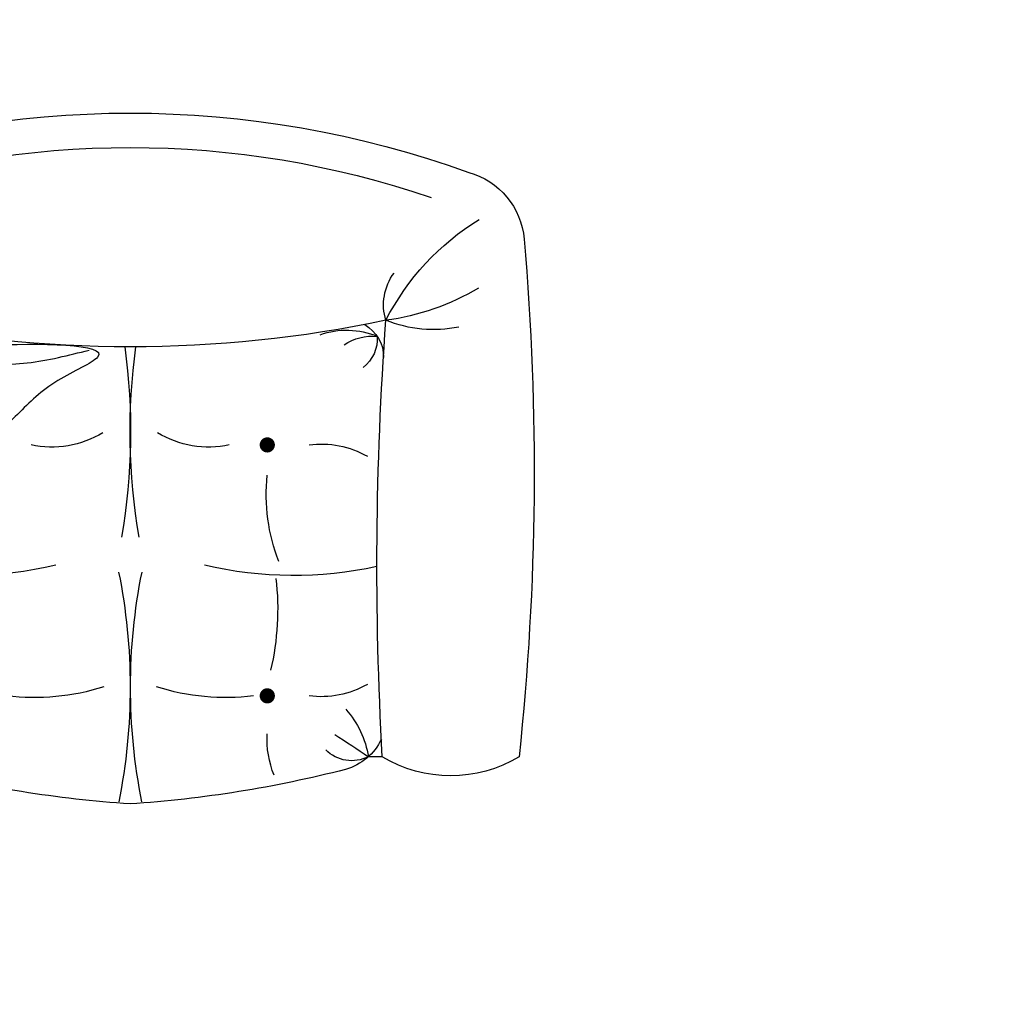
# Model space of a CAD drawing. Units: inches. Extents: x 844 to 2234, y 346 to 1084.
# Tile 23 of 93: x 1116 to 1136, y 710 to 731. Entities that reach past the tile are written whole.
import ezdxf

# ---------------------------------------------------------------- set-up
doc = ezdxf.new("R2010")
doc.units = ezdxf.units.IN
doc.header["$MEASUREMENT"] = 0
doc.layers.add('A-ANNO-DIMS', color=2, linetype='Continuous', lineweight=18)
doc.layers.add('furniture', color=8, linetype='Continuous', lineweight=18)
doc.layers.add('RA-AP-01$0$FURN', color=3, linetype='Continuous')
doc.layers.add('RA-AP-01$0$WOOD', color=64, linetype='Continuous')
doc.styles.get("Standard").update_dxf_attribs({"font": 'arial.ttf'})
doc.dimstyles.get("Standard").update_dxf_attribs({"dimtxt": 6, "dimasz": 3, "dimexe": 0.18, "dimexo": 0.0625, "dimgap": 0.09, "dimtad": 0, "dimtih": 1, "dimtoh": 1, "dimdec": 1, "dimzin": 0, "dimdsep": 46, "dimlunit": 3, "dimtxsty": 'Standard', "dimblk": 'ARCHTICK', "dimcen": 0.09, "dimadec": 0, "dimazin": 0, "dimtfac": 1, "dimtdec": 1, "dimtofl": 0, "dimtmove": 0, "dimatfit": 3, "dimfxl": 1, "dimtolj": 1, "dimtzin": 0, "dimarcsym": 0})

# ---------------------------------------------------------------- blocks, each defined once
blk = doc.blocks.new('A$C7F4351E2')
at = {"layer": 'RA-AP-01$0$FURN'}
for p, q in [((8.352559572600457, -8.263941955512525), (8.35255957259913, -8.282283310927069)), ((8.352559572600457, -8.927748273106442), (8.35255957259913, -8.909406917691898))]:
    blk.add_line(p, q, dxfattribs=at)
at = {"layer": 'RA-AP-01$0$FURN', "const_width": 0.01}
for points in [[(8.437812509519787, -8.415359762755768, 1), (8.427812509519786, -8.415359762755742, 1)], [(8.758197489244363, -8.415359762756214, -1), (8.768197489244365, -8.415359762756214, -1)], [(8.437812509519787, -8.776330465863198, -1), (8.427812509519786, -8.776330465863225, -1)], [(8.758197489244363, -8.776330465862753, 1), (8.768197489244365, -8.776330465862753, 1)]]:
    blk.add_lwpolyline(points, format="xyb", close=True, dxfattribs=at)
at = {"layer": 'RA-AP-01$0$FURN'}
for centre, radius, start, end in [((8.727559572604601, -11.61690445537682), 3.552808610866049, 85.0473312316413, 96.05887237565803), ((8.50205957259015, -8.17394195551301), 0.1744999999876311, 148.9517780040467, 211.048221995953), ((9.025650106946005, -8.176987401637472), 0.1, 15.499494600857, 85.04733123164159), ((8.77247054904813, -7.958543863781743), 0.3382138395168437, 297.2303327094027, 328.2563708342649), ((9.2484631175852, -8.302692737637487), 0.3241573581843151, 149.2985674842688, 172.3026350986055), ((7.88981694267423, -8.595845114309485), 1.310286319972027, 340.1192502251003, 19.8807497748998), ((9.084915705374858, -8.196040134964925), 0.1698955038956699, 168.877843135945, 201.8512383801196), ((7.929864357850293, -8.595845114309483), 1.224941341589781, 341.1257460634955, 18.87425393650447), ((8.947672844970796, -8.191835192646359), 0.0704710051510922, 253.1338634205325, 306.4126496157095), ((8.408522229993444, -8.33300072568355), 0.0753785023123622, 115.8745619060558, 163.9833547230034), ((8.603635103111959, -3.79706073025477), 4.473931917517753, 266.7828902523826, 274.1477233631118), ((8.878389979098333, -8.312202545234353), 0.05, 30.14777190425723, 89.99999999905349), ((10.52713941284929, -8.595845114309466), 1.634931324962266, 168.1200364254424, 191.8799635745573), ((9.101231010340802, -8.38034106221356), 0.5100538472773755, 167.6182489359307, 193.3122231353938), ((8.903279781571525, -8.31837865610295), 0.0478550828899777, 86.575295631534, 142.6833829238214), ((8.838100984994732, -8.276822957859652), 0.0683206773889159, 326.6729861493449, 5.218395042636973), ((8.810121490949696, -8.31110757721543), 0.1042084262671507, 340.4828318717155, 22.86929393278168), ((8.395364730619693, -8.304213854581548), 0.0479292786975047, 152.8070868543555, 225.4025460716553), ((8.333592787569726, -8.402663469525104), 0.1218651776285568, 48.0375529564433, 81.04623209541253), ((7.439612310514541, -8.913795367824825), 1.11020813118073, 31.93286085977143, 34.66647731879807), ((8.553131949433, -8.344109762755968), 0.1214118203512435, 150.1419074485596, 187.691663289156), ((8.642878049331348, -8.344109762756093), 0.1214118203512435, 352.3083367106845, 29.85809255128089), ((9.82633505008426, -8.696671375220811), 1.539060359583382, 165.5338783218257, 176.2437734318419), ((8.374918524725835, -8.294321202996931), 0.1212957045587361, 247.3375839744822, 273.7314750942433), ((8.546954810732721, -8.753394424755975), 0.3517162425384579, 83.41248966761125, 103.1674570565571), ((8.697701155637269, -8.172468128267624), 0.2442261434243043, 248.9017070735605, 275.9923925191661), ((8.73287643248165, -8.469775898206471), 0.3023568492824586, 173.0944825511667, 197.588060785551), ((8.889871101981017, -8.492307869305423), 0.1295083186917369, 167.9901339202812, 211.3796151021958), ((8.444145567704187, -7.829943385268752), 0.765467899454341, 258.6273206109321, 281.4174148186357), ((8.781211457338294, -7.772561243483908), 0.8232838708255751, 260.2449188973366, 277.7495311655964), ((9.82633505008426, -8.495018853398156), 1.539060359583382, 183.7562265681581, 194.4661216781742), ((8.444145567704187, -9.361312955433425), 0.765467899454341, 78.58258518136427, 101.3726793890678), ((8.781211457338294, -9.418695097218269), 0.8232838708255751, 82.25060502413102, 99.75508110266344), ((8.73287643248165, -8.721914330412496), 0.3023568492824586, 162.411939214449, 186.9055174488332), ((8.889871101981017, -8.699382359313544), 0.1295083186917369, 148.6203848978042, 192.0098660797188), ((9.101231010340802, -8.811349166405407), 0.5100538472773755, 166.6877768646062, 192.3817510640693), ((8.799643412436344, -8.749969313933361), 0.0689028341546707, 265.5384273543114, 353.5804828909086), ((8.374918524725835, -8.897369025622035), 0.1212957045587361, 86.26852490575668, 112.6624160255178), ((8.546954810732721, -8.438295803862992), 0.3517162425384579, 256.8325429434429, 276.5875103323888), ((8.697701155637269, -9.019222100351342), 0.2442261434243043, 84.00760748083387, 111.0982929264395), ((8.553131949433, -8.847580465862999), 0.1214118203512435, 172.308336710844, 209.8580925514404), ((8.785133372574222, -8.874256642962408), 0.0310151388417235, 42.62105484496073, 114.2239681486109), ((8.810121490949696, -8.880582651403534), 0.1042084262671507, 337.1307060672183, 19.51716812828453), ((8.395364730619693, -8.88747637403742), 0.0479292786975047, 134.5974539283447, 207.1929131456445), ((7.439612310514541, -8.277894860794142), 1.11020813118073, 325.333522681202, 328.0671391402286), ((8.838100984994732, -8.914867270759315), 0.0683206773889159, 354.781604957363, 33.32701385065517), ((8.408522229993444, -8.858689502935416), 0.0753785023123622, 196.0166452769965, 244.1254380939442), ((8.333592787569726, -8.789026759093863), 0.1218651776285568, 278.9537679045875, 311.9624470435567), ((8.642878049331348, -8.847580465862874), 0.1214118203512435, 330.1419074487191, 340.3913536181062), ((8.903279781571525, -8.873311572516016), 0.0478550828899777, 217.3166170761785, 273.424704368466), ((8.878389979098333, -8.879487683384612), 0.05, 270.0000000009465, 337.4173275753961), ((8.50205957259015, -9.017748273105955), 0.1744999999876311, 148.9517780040469, 211.0482219959533), ((8.603635103111959, -13.39462949836419), 4.473931917517753, 85.85227663688822, 93.21710974761734), ((8.947672844970796, -8.999855035972608), 0.0704710051510922, 53.58735038429053, 106.8661365794674), ((9.084915705374858, -8.995650093654042), 0.1698955038956699, 158.1487616198804, 191.122156864055), ((8.77247054904813, -9.233146364837223), 0.3382138395168437, 31.74362916573515, 62.76966729059727), ((9.2484631175852, -8.88899749098148), 0.3241573581843151, 187.6973649013944, 210.7014325157311), ((9.025650106946005, -9.014702826981493), 0.1, 274.9526687683584, 344.500505399143), ((8.727559572604601, -5.574785773242145), 3.552808610866049, 263.941127624342, 274.9526687683587)]:
    blk.add_arc(centre, radius, start, end, dxfattribs=at)
for points, knots in [([(8.764421239581775, -8.929562504990262), (8.755250524728652, -8.881106864374377), (8.74196437992213, -8.810906376383404), (8.80604948961138, -8.740469753734786), (8.847474678848357, -8.701097198289744), (8.897142214037096, -8.58322730303861), (8.897091569728207, -8.784804210134517), (8.88612504526093, -8.897825917224484), (8.806539053396843, -8.9185794820093), (8.764421239581775, -8.92956250499026)], [0, 0, 0, 0, 0.1367586589314792, 0.1981301758052368, 0.2677729570689282, 0.3281194902553322, 0.4737578340741565, 0.5765194025309516, 0.6920332287422236, 0.6920332287422236, 0.6920332287422236, 0.6920332287422236]), ([(8.764421239581775, -8.92956250499026), (8.782204778269502, -8.914603263160053), (8.821592007255505, -8.881471326160916), (8.86917941606436, -8.814322636989944), (8.867818990542759, -8.729338202119969), (8.881231406199264, -8.676770566934765), (8.888101821971249, -8.649843164808122)], [0, 0, 0, 0, 0.070018540671015, 0.1550780383534498, 0.2344491945777043, 0.3178048737568289, 0.3178048737568289, 0.3178048737568289, 0.3178048737568289])]:
    blk.add_open_spline(points, degree=3, knots=knots, dxfattribs=at)
blk = doc.blocks.new('A$C5D2F253E')
at = {"layer": 'RA-AP-01$0$WOOD', "xscale": -1, "rotation": 180}
blk.add_blockref('A$C7F4351E2', (-7.164808785335935, -7.45332973198748), dxfattribs=at)
blk = doc.blocks.new('_ArchTick')
at = {"color": 0, "linetype": 'ByBlock', "const_width": 0.15}
blk.add_lwpolyline([(-0.5, -0.5), (0.5, 0.5)], dxfattribs=at)
blk = doc.blocks.new('*D144')
at = {"layer": 'A-ANNO-DIMS', "color": 0, "lineweight": -2, "transparency": 16777216}
for p, q in [((1096.615948, 439.3732739999999), (1096.615948, 1074.743301)), ((1143.115948, 492.373274), (1143.115948, 1074.743301)), ((1096.615948, 1074.563301), (1102.481950728513, 1074.563301)), ((1143.115948, 1074.563301), (1137.249945271487, 1074.563301))]:
    blk.add_line(p, q, dxfattribs=at)
at = {"layer": 'Defpoints', "color": 0, "transparency": 16777216}
for p in [(1143.115948, 1074.563301), (1143.115948, 492.3107739999999), (1096.615948, 439.3107739999999)]:
    blk.add_point(p, dxfattribs=at)
at = {"layer": 'A-ANNO-DIMS', "color": 0, "lineweight": -2, "transparency": 16777216, "xscale": 3, "yscale": 3, "zscale": 3, "rotation": 180}
blk.add_blockref('_ArchTick', (1096.615948, 1074.563301), dxfattribs=at)
at = {"layer": 'A-ANNO-DIMS', "color": 0, "lineweight": -2, "transparency": 16777216, "xscale": 3, "yscale": 3, "zscale": 3}
blk.add_blockref('_ArchTick', (1143.115948, 1074.563301), dxfattribs=at)
at = {"layer": 'A-ANNO-DIMS', "color": 0, "transparency": 16777216, "insert": (1119.865948, 1074.563301), "char_height": 6, "attachment_point": 5}
blk.add_mtext('\\A1;3\'-10 1/2"', dxfattribs=at)

msp = doc.modelspace()

# ---------------------------------------------------------------- block references
at = {"layer": 'furniture', "xscale": 15.94108302203742, "yscale": 15.94108302203742, "zscale": 15.94108302203742, "rotation": 90}
msp.add_blockref('A$C5D2F253E', (1136.147844094663, 696.2584716700112), dxfattribs=at)

# ---------------------------------------------------------------- dimensions: what is measured, and where the dimension line sits
at = {"layer": 'A-ANNO-DIMS'}
dim = msp.add_linear_dim(base=(1143.115948, 1074.563301), p1=(1096.615948, 439.3107739999999), p2=(1143.115948, 492.3107739999999), dimstyle='Standard', override={"dimdec": 1, "dimlfac": 1, "dimrnd": 0, "dimzin": 1, "dimdsep": 46, "dimlunit": 4, "dimfrac": 2}, dxfattribs=at)
dim.commit()
dim.dimension.update_dxf_attribs({"geometry": '*D144', "text_midpoint": (1119.865948, 1074.563301)})

doc.saveas('drawing.dxf')
